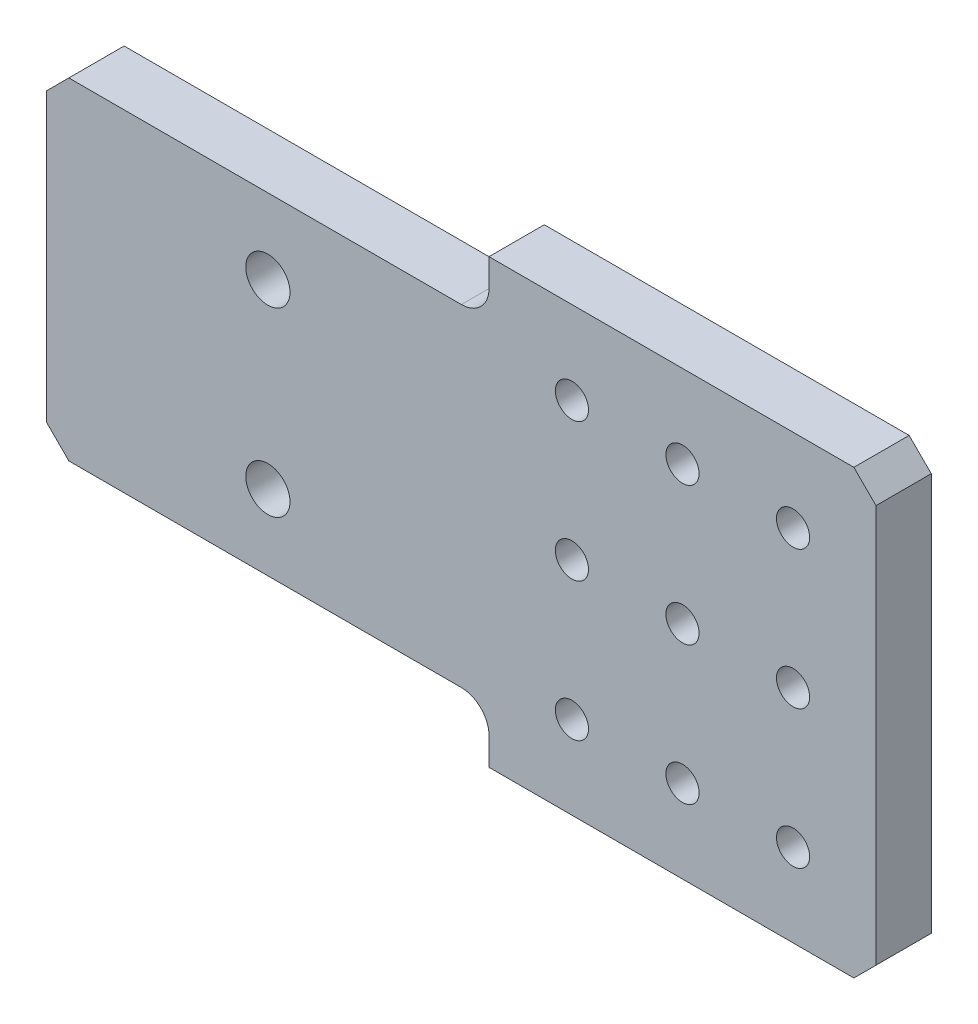
ISO-10303-21;
HEADER;
FILE_DESCRIPTION(('STEP AP214'),'2;1');
FILE_NAME('part.step','',(''),(''),'','','');
FILE_SCHEMA(('AUTOMOTIVE_DESIGN { 1 0 10303 214 1 1 1 1 }'));
ENDSEC;
DATA;
#1=APPLICATION_CONTEXT('core data for automotive mechanical design processes');
#2=APPLICATION_PROTOCOL_DEFINITION('international standard','automotive_design',2000,#1);
#3=PRODUCT_CONTEXT('',#1,'mechanical');
#4=PRODUCT('Part','Part','',(#3));
#5=PRODUCT_RELATED_PRODUCT_CATEGORY('part','',(#4));
#6=PRODUCT_DEFINITION_FORMATION('','',#4);
#7=PRODUCT_DEFINITION_CONTEXT('part definition',#1,'design');
#8=PRODUCT_DEFINITION('design','',#6,#7);
#9=PRODUCT_DEFINITION_SHAPE('','',#8);
#10=(LENGTH_UNIT() NAMED_UNIT(*) SI_UNIT(.MILLI.,.METRE.));
#11=(NAMED_UNIT(*) PLANE_ANGLE_UNIT() SI_UNIT($,.RADIAN.));
#12=(NAMED_UNIT(*) SI_UNIT($,.STERADIAN.) SOLID_ANGLE_UNIT());
#13=UNCERTAINTY_MEASURE_WITH_UNIT(LENGTH_MEASURE(1.E-05),#10,'distance_accuracy_value','');
#14=(GEOMETRIC_REPRESENTATION_CONTEXT(3) GLOBAL_UNCERTAINTY_ASSIGNED_CONTEXT((#13)) GLOBAL_UNIT_ASSIGNED_CONTEXT((#10,
#11,#12)) REPRESENTATION_CONTEXT('',''));
#15=CARTESIAN_POINT('',(0.,0.,0.));
#16=DIRECTION('',(0.,0.,1.));
#17=DIRECTION('',(1.,0.,0.));
#18=AXIS2_PLACEMENT_3D('',#15,#16,#17);
#19=CARTESIAN_POINT('',(3.75,1.75,0.5));
#20=DIRECTION('',(0.,0.,-1.));
#21=DIRECTION('',(-1.,0.,0.));
#22=AXIS2_PLACEMENT_3D('',#19,#20,#21);
#23=CYLINDRICAL_SURFACE('',#22,0.25);
#24=CARTESIAN_POINT('',(3.75,1.75,0.));
#25=DIRECTION('',(0.,0.,1.));
#26=DIRECTION('',(1.,0.,0.));
#27=AXIS2_PLACEMENT_3D('',#24,#25,#26);
#28=CIRCLE('',#27,0.25);
#29=CARTESIAN_POINT('',(3.75,1.5,0.));
#30=VERTEX_POINT('',#29);
#31=CARTESIAN_POINT('',(4.,1.75,0.));
#32=VERTEX_POINT('',#31);
#33=EDGE_CURVE('E168',#30,#32,#28,.T.);
#34=ORIENTED_EDGE('',*,*,#33,.F.);
#35=DIRECTION('',(0.,0.,-1.));
#36=VECTOR('',#35,1.);
#37=CARTESIAN_POINT('',(3.75,1.5,0.5));
#38=LINE('',#37,#36);
#39=CARTESIAN_POINT('',(3.75,1.5,0.5));
#40=VERTEX_POINT('',#39);
#41=EDGE_CURVE('E156',#40,#30,#38,.T.);
#42=ORIENTED_EDGE('',*,*,#41,.F.);
#43=CARTESIAN_POINT('',(3.75,1.75,0.5));
#44=DIRECTION('',(0.,0.,1.));
#45=DIRECTION('',(1.,0.,0.));
#46=AXIS2_PLACEMENT_3D('',#43,#44,#45);
#47=CIRCLE('',#46,0.25);
#48=CARTESIAN_POINT('',(4.,1.75,0.5));
#49=VERTEX_POINT('',#48);
#50=EDGE_CURVE('E163',#40,#49,#47,.T.);
#51=ORIENTED_EDGE('',*,*,#50,.T.);
#52=DIRECTION('',(0.,0.,-1.));
#53=VECTOR('',#52,1.);
#54=CARTESIAN_POINT('',(4.,1.75,0.5));
#55=LINE('',#54,#53);
#56=EDGE_CURVE('E201',#49,#32,#55,.T.);
#57=ORIENTED_EDGE('',*,*,#56,.T.);
#58=EDGE_LOOP('',(#34,#42,#51,#57));
#59=FACE_BOUND('',#58,.T.);
#60=ADVANCED_FACE('F47',(#59),#23,.F.);
#61=CARTESIAN_POINT('',(0.,1.5,0.5));
#62=DIRECTION('',(0.,1.,0.));
#63=DIRECTION('',(0.,0.,1.));
#64=AXIS2_PLACEMENT_3D('',#61,#62,#63);
#65=PLANE('',#64);
#66=DIRECTION('',(1.,0.,0.));
#67=VECTOR('',#66,1.);
#68=CARTESIAN_POINT('',(0.,1.5,0.));
#69=LINE('',#68,#67);
#70=CARTESIAN_POINT('',(0.199999999999999,1.5,0.));
#71=VERTEX_POINT('',#70);
#72=EDGE_CURVE('E202',#71,#30,#69,.T.);
#73=ORIENTED_EDGE('',*,*,#72,.F.);
#74=DIRECTION('',(0.,0.,1.));
#75=VECTOR('',#74,1.);
#76=CARTESIAN_POINT('',(0.199999999999999,1.5,0.5));
#77=LINE('',#76,#75);
#78=CARTESIAN_POINT('',(0.199999999999999,1.5,0.5));
#79=VERTEX_POINT('',#78);
#80=EDGE_CURVE('E157',#71,#79,#77,.T.);
#81=ORIENTED_EDGE('',*,*,#80,.T.);
#82=DIRECTION('',(1.,0.,0.));
#83=VECTOR('',#82,1.);
#84=CARTESIAN_POINT('',(0.,1.5,0.5));
#85=LINE('',#84,#83);
#86=EDGE_CURVE('E155',#79,#40,#85,.T.);
#87=ORIENTED_EDGE('',*,*,#86,.T.);
#88=ORIENTED_EDGE('',*,*,#41,.T.);
#89=EDGE_LOOP('',(#73,#81,#87,#88));
#90=FACE_BOUND('',#89,.T.);
#91=ADVANCED_FACE('F154',(#90),#65,.T.);
#92=CARTESIAN_POINT('',(0.,0.,0.5));
#93=DIRECTION('',(-1.,0.,0.));
#94=DIRECTION('',(0.,0.,1.));
#95=AXIS2_PLACEMENT_3D('',#92,#93,#94);
#96=PLANE('',#95);
#97=DIRECTION('',(0.,1.,0.));
#98=VECTOR('',#97,1.);
#99=CARTESIAN_POINT('',(0.,0.,0.));
#100=LINE('',#99,#98);
#101=CARTESIAN_POINT('',(0.,-1.3,0.));
#102=VERTEX_POINT('',#101);
#103=CARTESIAN_POINT('',(0.,1.3,0.));
#104=VERTEX_POINT('',#103);
#105=EDGE_CURVE('E208',#102,#104,#100,.T.);
#106=ORIENTED_EDGE('',*,*,#105,.F.);
#107=DIRECTION('',(0.,0.,1.));
#108=VECTOR('',#107,1.);
#109=CARTESIAN_POINT('',(0.,-1.3,0.5));
#110=LINE('',#109,#108);
#111=CARTESIAN_POINT('',(0.,-1.3,0.5));
#112=VERTEX_POINT('',#111);
#113=EDGE_CURVE('E11',#102,#112,#110,.T.);
#114=ORIENTED_EDGE('',*,*,#113,.T.);
#115=DIRECTION('',(0.,1.,0.));
#116=VECTOR('',#115,1.);
#117=CARTESIAN_POINT('',(0.,0.,0.5));
#118=LINE('',#117,#116);
#119=CARTESIAN_POINT('',(0.,1.3,0.5));
#120=VERTEX_POINT('',#119);
#121=EDGE_CURVE('E162',#112,#120,#118,.T.);
#122=ORIENTED_EDGE('',*,*,#121,.T.);
#123=DIRECTION('',(0.,0.,-1.));
#124=VECTOR('',#123,1.);
#125=CARTESIAN_POINT('',(0.,1.3,0.5));
#126=LINE('',#125,#124);
#127=EDGE_CURVE('E173',#120,#104,#126,.T.);
#128=ORIENTED_EDGE('',*,*,#127,.T.);
#129=EDGE_LOOP('',(#106,#114,#122,#128));
#130=FACE_BOUND('',#129,.T.);
#131=ADVANCED_FACE('F399',(#130),#96,.T.);
#132=CARTESIAN_POINT('',(0.,-1.5,0.5));
#133=DIRECTION('',(0.,1.,0.));
#134=DIRECTION('',(0.,0.,1.));
#135=AXIS2_PLACEMENT_3D('',#132,#133,#134);
#136=PLANE('',#135);
#137=DIRECTION('',(1.,0.,0.));
#138=VECTOR('',#137,1.);
#139=CARTESIAN_POINT('',(0.,-1.5,0.5));
#140=LINE('',#139,#138);
#141=CARTESIAN_POINT('',(0.200000000000001,-1.5,0.5));
#142=VERTEX_POINT('',#141);
#143=CARTESIAN_POINT('',(3.75,-1.5,0.5));
#144=VERTEX_POINT('',#143);
#145=EDGE_CURVE('E187',#142,#144,#140,.T.);
#146=ORIENTED_EDGE('',*,*,#145,.F.);
#147=DIRECTION('',(0.,0.,-1.));
#148=VECTOR('',#147,1.);
#149=CARTESIAN_POINT('',(0.200000000000001,-1.5,0.));
#150=LINE('',#149,#148);
#151=CARTESIAN_POINT('',(0.200000000000001,-1.5,0.));
#152=VERTEX_POINT('',#151);
#153=EDGE_CURVE('E56',#142,#152,#150,.T.);
#154=ORIENTED_EDGE('',*,*,#153,.T.);
#155=DIRECTION('',(1.,0.,0.));
#156=VECTOR('',#155,1.);
#157=CARTESIAN_POINT('',(0.,-1.5,0.));
#158=LINE('',#157,#156);
#159=CARTESIAN_POINT('',(3.75,-1.5,0.));
#160=VERTEX_POINT('',#159);
#161=EDGE_CURVE('E209',#152,#160,#158,.T.);
#162=ORIENTED_EDGE('',*,*,#161,.T.);
#163=DIRECTION('',(0.,0.,-1.));
#164=VECTOR('',#163,1.);
#165=CARTESIAN_POINT('',(3.75,-1.5,0.5));
#166=LINE('',#165,#164);
#167=EDGE_CURVE('E174',#144,#160,#166,.T.);
#168=ORIENTED_EDGE('',*,*,#167,.F.);
#169=EDGE_LOOP('',(#146,#154,#162,#168));
#170=FACE_BOUND('',#169,.T.);
#171=ADVANCED_FACE('F396',(#170),#136,.F.);
#172=CARTESIAN_POINT('',(3.75,-1.75,0.5));
#173=DIRECTION('',(0.,0.,-1.));
#174=DIRECTION('',(-1.,0.,0.));
#175=AXIS2_PLACEMENT_3D('',#172,#173,#174);
#176=CYLINDRICAL_SURFACE('',#175,0.25);
#177=CARTESIAN_POINT('',(3.75,-1.75,0.));
#178=DIRECTION('',(0.,0.,1.));
#179=DIRECTION('',(1.,0.,0.));
#180=AXIS2_PLACEMENT_3D('',#177,#178,#179);
#181=CIRCLE('',#180,0.25);
#182=CARTESIAN_POINT('',(4.,-1.75,0.));
#183=VERTEX_POINT('',#182);
#184=EDGE_CURVE('E215',#183,#160,#181,.T.);
#185=ORIENTED_EDGE('',*,*,#184,.F.);
#186=DIRECTION('',(0.,0.,-1.));
#187=VECTOR('',#186,1.);
#188=CARTESIAN_POINT('',(4.,-1.75,0.5));
#189=LINE('',#188,#187);
#190=CARTESIAN_POINT('',(4.,-1.75,0.5));
#191=VERTEX_POINT('',#190);
#192=EDGE_CURVE('E226',#191,#183,#189,.T.);
#193=ORIENTED_EDGE('',*,*,#192,.F.);
#194=CARTESIAN_POINT('',(3.75,-1.75,0.5));
#195=DIRECTION('',(0.,0.,1.));
#196=DIRECTION('',(1.,0.,0.));
#197=AXIS2_PLACEMENT_3D('',#194,#195,#196);
#198=CIRCLE('',#197,0.25);
#199=EDGE_CURVE('E186',#191,#144,#198,.T.);
#200=ORIENTED_EDGE('',*,*,#199,.T.);
#201=ORIENTED_EDGE('',*,*,#167,.T.);
#202=EDGE_LOOP('',(#185,#193,#200,#201));
#203=FACE_BOUND('',#202,.T.);
#204=ADVANCED_FACE('F392',(#203),#176,.F.);
#205=CARTESIAN_POINT('',(4.,0.,0.5));
#206=DIRECTION('',(1.,0.,0.));
#207=DIRECTION('',(0.,0.,-1.));
#208=AXIS2_PLACEMENT_3D('',#205,#206,#207);
#209=PLANE('',#208);
#210=DIRECTION('',(0.,-1.,0.));
#211=VECTOR('',#210,1.);
#212=CARTESIAN_POINT('',(4.,0.,0.));
#213=LINE('',#212,#211);
#214=CARTESIAN_POINT('',(4.,-2.,0.));
#215=VERTEX_POINT('',#214);
#216=EDGE_CURVE('E214',#183,#215,#213,.T.);
#217=ORIENTED_EDGE('',*,*,#216,.T.);
#218=DIRECTION('',(0.,0.,-1.));
#219=VECTOR('',#218,1.);
#220=CARTESIAN_POINT('',(4.,-2.,0.5));
#221=LINE('',#220,#219);
#222=CARTESIAN_POINT('',(4.,-2.,0.5));
#223=VERTEX_POINT('',#222);
#224=EDGE_CURVE('E229',#223,#215,#221,.T.);
#225=ORIENTED_EDGE('',*,*,#224,.F.);
#226=DIRECTION('',(0.,-1.,0.));
#227=VECTOR('',#226,1.);
#228=CARTESIAN_POINT('',(4.,0.,0.5));
#229=LINE('',#228,#227);
#230=EDGE_CURVE('E192',#191,#223,#229,.T.);
#231=ORIENTED_EDGE('',*,*,#230,.F.);
#232=ORIENTED_EDGE('',*,*,#192,.T.);
#233=EDGE_LOOP('',(#217,#225,#231,#232));
#234=FACE_BOUND('',#233,.T.);
#235=ADVANCED_FACE('F389',(#234),#209,.F.);
#236=CARTESIAN_POINT('',(0.,-2.,0.5));
#237=DIRECTION('',(0.,-1.,0.));
#238=DIRECTION('',(0.,0.,-1.));
#239=AXIS2_PLACEMENT_3D('',#236,#237,#238);
#240=PLANE('',#239);
#241=DIRECTION('',(-1.,0.,0.));
#242=VECTOR('',#241,1.);
#243=CARTESIAN_POINT('',(0.,-2.,0.));
#244=LINE('',#243,#242);
#245=CARTESIAN_POINT('',(7.3,-2.,0.));
#246=VERTEX_POINT('',#245);
#247=EDGE_CURVE('E217',#246,#215,#244,.T.);
#248=ORIENTED_EDGE('',*,*,#247,.F.);
#249=DIRECTION('',(0.,0.,1.));
#250=VECTOR('',#249,1.);
#251=CARTESIAN_POINT('',(7.3,-2.,0.5));
#252=LINE('',#251,#250);
#253=CARTESIAN_POINT('',(7.3,-2.,0.5));
#254=VERTEX_POINT('',#253);
#255=EDGE_CURVE('E259',#246,#254,#252,.T.);
#256=ORIENTED_EDGE('',*,*,#255,.T.);
#257=DIRECTION('',(-1.,0.,0.));
#258=VECTOR('',#257,1.);
#259=CARTESIAN_POINT('',(0.,-2.,0.5));
#260=LINE('',#259,#258);
#261=EDGE_CURVE('E198',#254,#223,#260,.T.);
#262=ORIENTED_EDGE('',*,*,#261,.T.);
#263=ORIENTED_EDGE('',*,*,#224,.T.);
#264=EDGE_LOOP('',(#248,#256,#262,#263));
#265=FACE_BOUND('',#264,.T.);
#266=ADVANCED_FACE('F382',(#265),#240,.T.);
#267=CARTESIAN_POINT('',(7.5,0.,0.5));
#268=DIRECTION('',(-1.,0.,0.));
#269=DIRECTION('',(0.,0.,1.));
#270=AXIS2_PLACEMENT_3D('',#267,#268,#269);
#271=PLANE('',#270);
#272=DIRECTION('',(0.,1.,0.));
#273=VECTOR('',#272,1.);
#274=CARTESIAN_POINT('',(7.5,0.,0.5));
#275=LINE('',#274,#273);
#276=CARTESIAN_POINT('',(7.5,-1.8,0.5));
#277=VERTEX_POINT('',#276);
#278=CARTESIAN_POINT('',(7.5,1.8,0.5));
#279=VERTEX_POINT('',#278);
#280=EDGE_CURVE('E196',#277,#279,#275,.T.);
#281=ORIENTED_EDGE('',*,*,#280,.F.);
#282=DIRECTION('',(0.,0.,-1.));
#283=VECTOR('',#282,1.);
#284=CARTESIAN_POINT('',(7.5,-1.8,0.));
#285=LINE('',#284,#283);
#286=CARTESIAN_POINT('',(7.5,-1.8,0.));
#287=VERTEX_POINT('',#286);
#288=EDGE_CURVE('E252',#277,#287,#285,.T.);
#289=ORIENTED_EDGE('',*,*,#288,.T.);
#290=DIRECTION('',(0.,1.,0.));
#291=VECTOR('',#290,1.);
#292=CARTESIAN_POINT('',(7.5,0.,0.));
#293=LINE('',#292,#291);
#294=CARTESIAN_POINT('',(7.5,1.8,0.));
#295=VERTEX_POINT('',#294);
#296=EDGE_CURVE('E219',#287,#295,#293,.T.);
#297=ORIENTED_EDGE('',*,*,#296,.T.);
#298=DIRECTION('',(0.,0.,1.));
#299=VECTOR('',#298,1.);
#300=CARTESIAN_POINT('',(7.5,1.8,0.5));
#301=LINE('',#300,#299);
#302=EDGE_CURVE('E248',#295,#279,#301,.T.);
#303=ORIENTED_EDGE('',*,*,#302,.T.);
#304=EDGE_LOOP('',(#281,#289,#297,#303));
#305=FACE_BOUND('',#304,.T.);
#306=ADVANCED_FACE('F374',(#305),#271,.F.);
#307=CARTESIAN_POINT('',(0.,2.,0.5));
#308=DIRECTION('',(0.,-1.,0.));
#309=DIRECTION('',(0.,0.,-1.));
#310=AXIS2_PLACEMENT_3D('',#307,#308,#309);
#311=PLANE('',#310);
#312=DIRECTION('',(-1.,0.,0.));
#313=VECTOR('',#312,1.);
#314=CARTESIAN_POINT('',(0.,2.,0.5));
#315=LINE('',#314,#313);
#316=CARTESIAN_POINT('',(7.3,2.,0.5));
#317=VERTEX_POINT('',#316);
#318=CARTESIAN_POINT('',(4.,2.,0.5));
#319=VERTEX_POINT('',#318);
#320=EDGE_CURVE('E199',#317,#319,#315,.T.);
#321=ORIENTED_EDGE('',*,*,#320,.F.);
#322=DIRECTION('',(0.,0.,-1.));
#323=VECTOR('',#322,1.);
#324=CARTESIAN_POINT('',(7.3,2.,0.5));
#325=LINE('',#324,#323);
#326=CARTESIAN_POINT('',(7.3,2.,0.));
#327=VERTEX_POINT('',#326);
#328=EDGE_CURVE('E246',#317,#327,#325,.T.);
#329=ORIENTED_EDGE('',*,*,#328,.T.);
#330=DIRECTION('',(-1.,0.,0.));
#331=VECTOR('',#330,1.);
#332=CARTESIAN_POINT('',(0.,2.,0.));
#333=LINE('',#332,#331);
#334=CARTESIAN_POINT('',(4.,2.,0.));
#335=VERTEX_POINT('',#334);
#336=EDGE_CURVE('E182',#327,#335,#333,.T.);
#337=ORIENTED_EDGE('',*,*,#336,.T.);
#338=DIRECTION('',(0.,0.,-1.));
#339=VECTOR('',#338,1.);
#340=CARTESIAN_POINT('',(4.,2.,0.5));
#341=LINE('',#340,#339);
#342=EDGE_CURVE('E221',#319,#335,#341,.T.);
#343=ORIENTED_EDGE('',*,*,#342,.F.);
#344=EDGE_LOOP('',(#321,#329,#337,#343));
#345=FACE_BOUND('',#344,.T.);
#346=ADVANCED_FACE('F439',(#345),#311,.F.);
#347=CARTESIAN_POINT('',(4.,0.,0.5));
#348=DIRECTION('',(-1.,0.,0.));
#349=DIRECTION('',(0.,0.,1.));
#350=AXIS2_PLACEMENT_3D('',#347,#348,#349);
#351=PLANE('',#350);
#352=DIRECTION('',(0.,1.,0.));
#353=VECTOR('',#352,1.);
#354=CARTESIAN_POINT('',(4.,0.,0.));
#355=LINE('',#354,#353);
#356=EDGE_CURVE('E177',#32,#335,#355,.T.);
#357=ORIENTED_EDGE('',*,*,#356,.F.);
#358=ORIENTED_EDGE('',*,*,#56,.F.);
#359=DIRECTION('',(0.,1.,0.));
#360=VECTOR('',#359,1.);
#361=CARTESIAN_POINT('',(4.,0.,0.5));
#362=LINE('',#361,#360);
#363=EDGE_CURVE('E180',#49,#319,#362,.T.);
#364=ORIENTED_EDGE('',*,*,#363,.T.);
#365=ORIENTED_EDGE('',*,*,#342,.T.);
#366=EDGE_LOOP('',(#357,#358,#364,#365));
#367=FACE_BOUND('',#366,.T.);
#368=ADVANCED_FACE('F336',(#367),#351,.T.);
#369=CARTESIAN_POINT('',(0.,0.,0.5));
#370=DIRECTION('',(0.,0.,1.));
#371=DIRECTION('',(1.,0.,0.));
#372=AXIS2_PLACEMENT_3D('',#369,#370,#371);
#373=PLANE('',#372);
#374=CARTESIAN_POINT('',(5.75,1.25,0.5));
#375=DIRECTION('',(0.,0.,1.));
#376=DIRECTION('',(1.,0.,0.));
#377=AXIS2_PLACEMENT_3D('',#374,#375,#376);
#378=CIRCLE('',#377,0.15);
#379=CARTESIAN_POINT('',(5.9,1.25,0.5));
#380=VERTEX_POINT('',#379);
#381=EDGE_CURVE('E310',#380,#380,#378,.T.);
#382=ORIENTED_EDGE('',*,*,#381,.F.);
#383=EDGE_LOOP('',(#382));
#384=FACE_BOUND('',#383,.T.);
#385=CARTESIAN_POINT('',(6.75,1.25,0.5));
#386=DIRECTION('',(0.,0.,1.));
#387=DIRECTION('',(1.,0.,0.));
#388=AXIS2_PLACEMENT_3D('',#385,#386,#387);
#389=CIRCLE('',#388,0.15);
#390=CARTESIAN_POINT('',(6.9,1.25,0.5));
#391=VERTEX_POINT('',#390);
#392=EDGE_CURVE('E320',#391,#391,#389,.T.);
#393=ORIENTED_EDGE('',*,*,#392,.F.);
#394=EDGE_LOOP('',(#393));
#395=FACE_BOUND('',#394,.T.);
#396=CARTESIAN_POINT('',(6.75,0.,0.5));
#397=DIRECTION('',(0.,0.,1.));
#398=DIRECTION('',(1.,0.,0.));
#399=AXIS2_PLACEMENT_3D('',#396,#397,#398);
#400=CIRCLE('',#399,0.15);
#401=CARTESIAN_POINT('',(6.9,0.,0.5));
#402=VERTEX_POINT('',#401);
#403=EDGE_CURVE('E311',#402,#402,#400,.T.);
#404=ORIENTED_EDGE('',*,*,#403,.F.);
#405=EDGE_LOOP('',(#404));
#406=FACE_BOUND('',#405,.T.);
#407=CARTESIAN_POINT('',(6.75,-1.25,0.5));
#408=DIRECTION('',(0.,0.,1.));
#409=DIRECTION('',(1.,0.,0.));
#410=AXIS2_PLACEMENT_3D('',#407,#408,#409);
#411=CIRCLE('',#410,0.15);
#412=CARTESIAN_POINT('',(6.9,-1.25,0.5));
#413=VERTEX_POINT('',#412);
#414=EDGE_CURVE('E309',#413,#413,#411,.T.);
#415=ORIENTED_EDGE('',*,*,#414,.F.);
#416=EDGE_LOOP('',(#415));
#417=FACE_BOUND('',#416,.T.);
#418=CARTESIAN_POINT('',(5.75,-1.25,0.5));
#419=DIRECTION('',(0.,0.,1.));
#420=DIRECTION('',(1.,0.,0.));
#421=AXIS2_PLACEMENT_3D('',#418,#419,#420);
#422=CIRCLE('',#421,0.15);
#423=CARTESIAN_POINT('',(5.9,-1.25,0.5));
#424=VERTEX_POINT('',#423);
#425=EDGE_CURVE('E314',#424,#424,#422,.T.);
#426=ORIENTED_EDGE('',*,*,#425,.F.);
#427=EDGE_LOOP('',(#426));
#428=FACE_BOUND('',#427,.T.);
#429=CARTESIAN_POINT('',(4.75,-1.25,0.5));
#430=DIRECTION('',(0.,0.,1.));
#431=DIRECTION('',(1.,0.,0.));
#432=AXIS2_PLACEMENT_3D('',#429,#430,#431);
#433=CIRCLE('',#432,0.15);
#434=CARTESIAN_POINT('',(4.9,-1.25,0.5));
#435=VERTEX_POINT('',#434);
#436=EDGE_CURVE('E327',#435,#435,#433,.T.);
#437=ORIENTED_EDGE('',*,*,#436,.F.);
#438=EDGE_LOOP('',(#437));
#439=FACE_BOUND('',#438,.T.);
#440=CARTESIAN_POINT('',(4.75,0.,0.5));
#441=DIRECTION('',(0.,0.,1.));
#442=DIRECTION('',(1.,0.,0.));
#443=AXIS2_PLACEMENT_3D('',#440,#441,#442);
#444=CIRCLE('',#443,0.15);
#445=CARTESIAN_POINT('',(4.9,0.,0.5));
#446=VERTEX_POINT('',#445);
#447=EDGE_CURVE('E324',#446,#446,#444,.T.);
#448=ORIENTED_EDGE('',*,*,#447,.F.);
#449=EDGE_LOOP('',(#448));
#450=FACE_BOUND('',#449,.T.);
#451=CARTESIAN_POINT('',(5.75,0.,0.5));
#452=DIRECTION('',(0.,0.,1.));
#453=DIRECTION('',(1.,0.,0.));
#454=AXIS2_PLACEMENT_3D('',#451,#452,#453);
#455=CIRCLE('',#454,0.15);
#456=CARTESIAN_POINT('',(5.9,0.,0.5));
#457=VERTEX_POINT('',#456);
#458=EDGE_CURVE('E325',#457,#457,#455,.T.);
#459=ORIENTED_EDGE('',*,*,#458,.F.);
#460=EDGE_LOOP('',(#459));
#461=FACE_BOUND('',#460,.T.);
#462=CARTESIAN_POINT('',(4.75,1.25,0.5));
#463=DIRECTION('',(0.,0.,1.));
#464=DIRECTION('',(1.,0.,0.));
#465=AXIS2_PLACEMENT_3D('',#462,#463,#464);
#466=CIRCLE('',#465,0.15);
#467=CARTESIAN_POINT('',(4.9,1.25,0.5));
#468=VERTEX_POINT('',#467);
#469=EDGE_CURVE('E277',#468,#468,#466,.T.);
#470=ORIENTED_EDGE('',*,*,#469,.F.);
#471=EDGE_LOOP('',(#470));
#472=FACE_BOUND('',#471,.T.);
#473=CARTESIAN_POINT('',(2.,0.82,0.5));
#474=DIRECTION('',(0.,0.,1.));
#475=DIRECTION('',(1.,0.,0.));
#476=AXIS2_PLACEMENT_3D('',#473,#474,#475);
#477=CIRCLE('',#476,0.2);
#478=CARTESIAN_POINT('',(2.2,0.82,0.5));
#479=VERTEX_POINT('',#478);
#480=EDGE_CURVE('E267',#479,#479,#477,.T.);
#481=ORIENTED_EDGE('',*,*,#480,.F.);
#482=EDGE_LOOP('',(#481));
#483=FACE_BOUND('',#482,.T.);
#484=CARTESIAN_POINT('',(2.,-0.82,0.5));
#485=DIRECTION('',(0.,0.,1.));
#486=DIRECTION('',(1.,0.,0.));
#487=AXIS2_PLACEMENT_3D('',#484,#485,#486);
#488=CIRCLE('',#487,0.2);
#489=CARTESIAN_POINT('',(2.2,-0.82,0.5));
#490=VERTEX_POINT('',#489);
#491=EDGE_CURVE('E184',#490,#490,#488,.T.);
#492=ORIENTED_EDGE('',*,*,#491,.F.);
#493=EDGE_LOOP('',(#492));
#494=FACE_BOUND('',#493,.T.);
#495=ORIENTED_EDGE('',*,*,#261,.F.);
#496=DIRECTION('',(0.707106781186549,0.707106781186546,0.));
#497=VECTOR('',#496,1.);
#498=CARTESIAN_POINT('',(4.64999999999998,-4.65,0.5));
#499=LINE('',#498,#497);
#500=EDGE_CURVE('E265',#254,#277,#499,.T.);
#501=ORIENTED_EDGE('',*,*,#500,.T.);
#502=ORIENTED_EDGE('',*,*,#280,.T.);
#503=DIRECTION('',(0.707106781186546,-0.707106781186549,0.));
#504=VECTOR('',#503,1.);
#505=CARTESIAN_POINT('',(4.65000000000002,4.65,0.5));
#506=LINE('',#505,#504);
#507=EDGE_CURVE('E244',#279,#317,#506,.F.);
#508=ORIENTED_EDGE('',*,*,#507,.T.);
#509=ORIENTED_EDGE('',*,*,#320,.T.);
#510=ORIENTED_EDGE('',*,*,#363,.F.);
#511=ORIENTED_EDGE('',*,*,#50,.F.);
#512=ORIENTED_EDGE('',*,*,#86,.F.);
#513=DIRECTION('',(0.707106781186548,0.707106781186548,0.));
#514=VECTOR('',#513,1.);
#515=CARTESIAN_POINT('',(-0.65,0.65,0.5));
#516=LINE('',#515,#514);
#517=EDGE_CURVE('E245',#79,#120,#516,.F.);
#518=ORIENTED_EDGE('',*,*,#517,.T.);
#519=ORIENTED_EDGE('',*,*,#121,.F.);
#520=DIRECTION('',(0.707106781186546,-0.707106781186549,0.));
#521=VECTOR('',#520,1.);
#522=CARTESIAN_POINT('',(-0.649999999999999,-0.649999999999997,0.5));
#523=LINE('',#522,#521);
#524=EDGE_CURVE('E70',#112,#142,#523,.T.);
#525=ORIENTED_EDGE('',*,*,#524,.T.);
#526=ORIENTED_EDGE('',*,*,#145,.T.);
#527=ORIENTED_EDGE('',*,*,#199,.F.);
#528=ORIENTED_EDGE('',*,*,#230,.T.);
#529=EDGE_LOOP('',(#495,#501,#502,#508,#509,#510,#511,#512,#518,#519,#525,#526,#527,#528));
#530=FACE_BOUND('',#529,.T.);
#531=ADVANCED_FACE('F171',(#384,#395,#406,#417,#428,#439,#450,#461,#472,#483,#494,#530),#373,.T.);
#532=CARTESIAN_POINT('',(0.,0.,0.));
#533=DIRECTION('',(0.,0.,1.));
#534=DIRECTION('',(1.,0.,0.));
#535=AXIS2_PLACEMENT_3D('',#532,#533,#534);
#536=PLANE('',#535);
#537=CARTESIAN_POINT('',(5.75,1.25,0.));
#538=DIRECTION('',(0.,0.,1.));
#539=DIRECTION('',(1.,0.,0.));
#540=AXIS2_PLACEMENT_3D('',#537,#538,#539);
#541=CIRCLE('',#540,0.15);
#542=CARTESIAN_POINT('',(5.9,1.25,0.));
#543=VERTEX_POINT('',#542);
#544=EDGE_CURVE('E53',#543,#543,#541,.T.);
#545=ORIENTED_EDGE('',*,*,#544,.T.);
#546=EDGE_LOOP('',(#545));
#547=FACE_BOUND('',#546,.T.);
#548=CARTESIAN_POINT('',(6.75,1.25,0.));
#549=DIRECTION('',(0.,0.,1.));
#550=DIRECTION('',(1.,0.,0.));
#551=AXIS2_PLACEMENT_3D('',#548,#549,#550);
#552=CIRCLE('',#551,0.15);
#553=CARTESIAN_POINT('',(6.9,1.25,0.));
#554=VERTEX_POINT('',#553);
#555=EDGE_CURVE('E291',#554,#554,#552,.T.);
#556=ORIENTED_EDGE('',*,*,#555,.T.);
#557=EDGE_LOOP('',(#556));
#558=FACE_BOUND('',#557,.T.);
#559=CARTESIAN_POINT('',(6.75,0.,0.));
#560=DIRECTION('',(0.,0.,1.));
#561=DIRECTION('',(1.,0.,0.));
#562=AXIS2_PLACEMENT_3D('',#559,#560,#561);
#563=CIRCLE('',#562,0.15);
#564=CARTESIAN_POINT('',(6.9,0.,0.));
#565=VERTEX_POINT('',#564);
#566=EDGE_CURVE('E292',#565,#565,#563,.T.);
#567=ORIENTED_EDGE('',*,*,#566,.T.);
#568=EDGE_LOOP('',(#567));
#569=FACE_BOUND('',#568,.T.);
#570=CARTESIAN_POINT('',(6.75,-1.25,0.));
#571=DIRECTION('',(0.,0.,1.));
#572=DIRECTION('',(1.,0.,0.));
#573=AXIS2_PLACEMENT_3D('',#570,#571,#572);
#574=CIRCLE('',#573,0.15);
#575=CARTESIAN_POINT('',(6.9,-1.25,0.));
#576=VERTEX_POINT('',#575);
#577=EDGE_CURVE('E287',#576,#576,#574,.T.);
#578=ORIENTED_EDGE('',*,*,#577,.T.);
#579=EDGE_LOOP('',(#578));
#580=FACE_BOUND('',#579,.T.);
#581=CARTESIAN_POINT('',(5.75,-1.25,0.));
#582=DIRECTION('',(0.,0.,1.));
#583=DIRECTION('',(1.,0.,0.));
#584=AXIS2_PLACEMENT_3D('',#581,#582,#583);
#585=CIRCLE('',#584,0.15);
#586=CARTESIAN_POINT('',(5.9,-1.25,0.));
#587=VERTEX_POINT('',#586);
#588=EDGE_CURVE('E281',#587,#587,#585,.T.);
#589=ORIENTED_EDGE('',*,*,#588,.T.);
#590=EDGE_LOOP('',(#589));
#591=FACE_BOUND('',#590,.T.);
#592=CARTESIAN_POINT('',(4.75,-1.25,0.));
#593=DIRECTION('',(0.,0.,1.));
#594=DIRECTION('',(1.,0.,0.));
#595=AXIS2_PLACEMENT_3D('',#592,#593,#594);
#596=CIRCLE('',#595,0.15);
#597=CARTESIAN_POINT('',(4.9,-1.25,0.));
#598=VERTEX_POINT('',#597);
#599=EDGE_CURVE('E284',#598,#598,#596,.T.);
#600=ORIENTED_EDGE('',*,*,#599,.T.);
#601=EDGE_LOOP('',(#600));
#602=FACE_BOUND('',#601,.T.);
#603=CARTESIAN_POINT('',(4.75,0.,0.));
#604=DIRECTION('',(0.,0.,1.));
#605=DIRECTION('',(1.,0.,0.));
#606=AXIS2_PLACEMENT_3D('',#603,#604,#605);
#607=CIRCLE('',#606,0.15);
#608=CARTESIAN_POINT('',(4.9,0.,0.));
#609=VERTEX_POINT('',#608);
#610=EDGE_CURVE('E276',#609,#609,#607,.T.);
#611=ORIENTED_EDGE('',*,*,#610,.T.);
#612=EDGE_LOOP('',(#611));
#613=FACE_BOUND('',#612,.T.);
#614=CARTESIAN_POINT('',(5.75,0.,0.));
#615=DIRECTION('',(0.,0.,1.));
#616=DIRECTION('',(1.,0.,0.));
#617=AXIS2_PLACEMENT_3D('',#614,#615,#616);
#618=CIRCLE('',#617,0.15);
#619=CARTESIAN_POINT('',(5.9,0.,0.));
#620=VERTEX_POINT('',#619);
#621=EDGE_CURVE('E274',#620,#620,#618,.T.);
#622=ORIENTED_EDGE('',*,*,#621,.T.);
#623=EDGE_LOOP('',(#622));
#624=FACE_BOUND('',#623,.T.);
#625=CARTESIAN_POINT('',(4.75,1.25,0.));
#626=DIRECTION('',(0.,0.,1.));
#627=DIRECTION('',(1.,0.,0.));
#628=AXIS2_PLACEMENT_3D('',#625,#626,#627);
#629=CIRCLE('',#628,0.15);
#630=CARTESIAN_POINT('',(4.9,1.25,0.));
#631=VERTEX_POINT('',#630);
#632=EDGE_CURVE('E275',#631,#631,#629,.T.);
#633=ORIENTED_EDGE('',*,*,#632,.T.);
#634=EDGE_LOOP('',(#633));
#635=FACE_BOUND('',#634,.T.);
#636=CARTESIAN_POINT('',(2.,0.82,0.));
#637=DIRECTION('',(0.,0.,1.));
#638=DIRECTION('',(1.,0.,0.));
#639=AXIS2_PLACEMENT_3D('',#636,#637,#638);
#640=CIRCLE('',#639,0.2);
#641=CARTESIAN_POINT('',(2.2,0.82,0.));
#642=VERTEX_POINT('',#641);
#643=EDGE_CURVE('E206',#642,#642,#640,.T.);
#644=ORIENTED_EDGE('',*,*,#643,.T.);
#645=EDGE_LOOP('',(#644));
#646=FACE_BOUND('',#645,.T.);
#647=CARTESIAN_POINT('',(2.,-0.82,0.));
#648=DIRECTION('',(0.,0.,1.));
#649=DIRECTION('',(1.,0.,0.));
#650=AXIS2_PLACEMENT_3D('',#647,#648,#649);
#651=CIRCLE('',#650,0.2);
#652=CARTESIAN_POINT('',(2.2,-0.82,0.));
#653=VERTEX_POINT('',#652);
#654=EDGE_CURVE('E266',#653,#653,#651,.T.);
#655=ORIENTED_EDGE('',*,*,#654,.T.);
#656=EDGE_LOOP('',(#655));
#657=FACE_BOUND('',#656,.T.);
#658=ORIENTED_EDGE('',*,*,#296,.F.);
#659=DIRECTION('',(-0.707106781186549,-0.707106781186546,0.));
#660=VECTOR('',#659,1.);
#661=CARTESIAN_POINT('',(7.5,-1.8,0.));
#662=LINE('',#661,#660);
#663=EDGE_CURVE('E260',#287,#246,#662,.T.);
#664=ORIENTED_EDGE('',*,*,#663,.T.);
#665=ORIENTED_EDGE('',*,*,#247,.T.);
#666=ORIENTED_EDGE('',*,*,#216,.F.);
#667=ORIENTED_EDGE('',*,*,#184,.T.);
#668=ORIENTED_EDGE('',*,*,#161,.F.);
#669=DIRECTION('',(-0.707106781186546,0.707106781186549,0.));
#670=VECTOR('',#669,1.);
#671=CARTESIAN_POINT('',(0.200000000000001,-1.5,0.));
#672=LINE('',#671,#670);
#673=EDGE_CURVE('E254',#152,#102,#672,.T.);
#674=ORIENTED_EDGE('',*,*,#673,.T.);
#675=ORIENTED_EDGE('',*,*,#105,.T.);
#676=DIRECTION('',(-0.707106781186548,-0.707106781186548,0.));
#677=VECTOR('',#676,1.);
#678=CARTESIAN_POINT('',(0.,1.3,0.));
#679=LINE('',#678,#677);
#680=EDGE_CURVE('E239',#104,#71,#679,.F.);
#681=ORIENTED_EDGE('',*,*,#680,.T.);
#682=ORIENTED_EDGE('',*,*,#72,.T.);
#683=ORIENTED_EDGE('',*,*,#33,.T.);
#684=ORIENTED_EDGE('',*,*,#356,.T.);
#685=ORIENTED_EDGE('',*,*,#336,.F.);
#686=DIRECTION('',(-0.707106781186546,0.707106781186549,0.));
#687=VECTOR('',#686,1.);
#688=CARTESIAN_POINT('',(7.3,2.,0.));
#689=LINE('',#688,#687);
#690=EDGE_CURVE('E237',#327,#295,#689,.F.);
#691=ORIENTED_EDGE('',*,*,#690,.T.);
#692=EDGE_LOOP('',(#658,#664,#665,#666,#667,#668,#674,#675,#681,#682,#683,#684,#685,#691));
#693=FACE_BOUND('',#692,.T.);
#694=ADVANCED_FACE('F340',(#547,#558,#569,#580,#591,#602,#613,#624,#635,#646,#657,#693),#536,.F.);
#695=CARTESIAN_POINT('',(0.,1.3,0.5));
#696=DIRECTION('',(0.707106781186548,-0.707106781186548,0.));
#697=DIRECTION('',(0.,0.,-1.));
#698=AXIS2_PLACEMENT_3D('',#695,#696,#697);
#699=PLANE('',#698);
#700=ORIENTED_EDGE('',*,*,#517,.F.);
#701=ORIENTED_EDGE('',*,*,#80,.F.);
#702=ORIENTED_EDGE('',*,*,#680,.F.);
#703=ORIENTED_EDGE('',*,*,#127,.F.);
#704=EDGE_LOOP('',(#700,#701,#702,#703));
#705=FACE_BOUND('',#704,.T.);
#706=ADVANCED_FACE('F361',(#705),#699,.F.);
#707=CARTESIAN_POINT('',(7.3,2.,0.5));
#708=DIRECTION('',(-0.707106781186549,-0.707106781186546,0.));
#709=DIRECTION('',(0.,0.,-1.));
#710=AXIS2_PLACEMENT_3D('',#707,#708,#709);
#711=PLANE('',#710);
#712=ORIENTED_EDGE('',*,*,#507,.F.);
#713=ORIENTED_EDGE('',*,*,#302,.F.);
#714=ORIENTED_EDGE('',*,*,#690,.F.);
#715=ORIENTED_EDGE('',*,*,#328,.F.);
#716=EDGE_LOOP('',(#712,#713,#714,#715));
#717=FACE_BOUND('',#716,.T.);
#718=ADVANCED_FACE('F410',(#717),#711,.F.);
#719=CARTESIAN_POINT('',(7.5,-1.8,0.5));
#720=DIRECTION('',(0.707106781186546,-0.707106781186549,0.));
#721=DIRECTION('',(0.,0.,1.));
#722=AXIS2_PLACEMENT_3D('',#719,#720,#721);
#723=PLANE('',#722);
#724=ORIENTED_EDGE('',*,*,#500,.F.);
#725=ORIENTED_EDGE('',*,*,#255,.F.);
#726=ORIENTED_EDGE('',*,*,#663,.F.);
#727=ORIENTED_EDGE('',*,*,#288,.F.);
#728=EDGE_LOOP('',(#724,#725,#726,#727));
#729=FACE_BOUND('',#728,.T.);
#730=ADVANCED_FACE('F379',(#729),#723,.T.);
#731=CARTESIAN_POINT('',(0.200000000000001,-1.5,0.5));
#732=DIRECTION('',(-0.707106781186549,-0.707106781186546,0.));
#733=DIRECTION('',(0.,0.,1.));
#734=AXIS2_PLACEMENT_3D('',#731,#732,#733);
#735=PLANE('',#734);
#736=ORIENTED_EDGE('',*,*,#524,.F.);
#737=ORIENTED_EDGE('',*,*,#113,.F.);
#738=ORIENTED_EDGE('',*,*,#673,.F.);
#739=ORIENTED_EDGE('',*,*,#153,.F.);
#740=EDGE_LOOP('',(#736,#737,#738,#739));
#741=FACE_BOUND('',#740,.T.);
#742=ADVANCED_FACE('F55',(#741),#735,.T.);
#743=CARTESIAN_POINT('',(2.,-0.82,-0.5));
#744=DIRECTION('',(0.,0.,1.));
#745=DIRECTION('',(1.,0.,0.));
#746=AXIS2_PLACEMENT_3D('',#743,#744,#745);
#747=CYLINDRICAL_SURFACE('',#746,0.2);
#748=ORIENTED_EDGE('',*,*,#491,.T.);
#749=EDGE_LOOP('',(#748));
#750=FACE_BOUND('',#749,.T.);
#751=ORIENTED_EDGE('',*,*,#654,.F.);
#752=EDGE_LOOP('',(#751));
#753=FACE_BOUND('',#752,.T.);
#754=ADVANCED_FACE('F401',(#750,#753),#747,.F.);
#755=CARTESIAN_POINT('',(2.,0.82,-0.5));
#756=DIRECTION('',(0.,0.,1.));
#757=DIRECTION('',(1.,0.,0.));
#758=AXIS2_PLACEMENT_3D('',#755,#756,#757);
#759=CYLINDRICAL_SURFACE('',#758,0.2);
#760=ORIENTED_EDGE('',*,*,#480,.T.);
#761=EDGE_LOOP('',(#760));
#762=FACE_BOUND('',#761,.T.);
#763=ORIENTED_EDGE('',*,*,#643,.F.);
#764=EDGE_LOOP('',(#763));
#765=FACE_BOUND('',#764,.T.);
#766=ADVANCED_FACE('F360',(#762,#765),#759,.F.);
#767=CARTESIAN_POINT('',(4.75,1.25,-0.5));
#768=DIRECTION('',(0.,0.,1.));
#769=DIRECTION('',(1.,0.,0.));
#770=AXIS2_PLACEMENT_3D('',#767,#768,#769);
#771=CYLINDRICAL_SURFACE('',#770,0.15);
#772=ORIENTED_EDGE('',*,*,#469,.T.);
#773=EDGE_LOOP('',(#772));
#774=FACE_BOUND('',#773,.T.);
#775=ORIENTED_EDGE('',*,*,#632,.F.);
#776=EDGE_LOOP('',(#775));
#777=FACE_BOUND('',#776,.T.);
#778=ADVANCED_FACE('F352',(#774,#777),#771,.F.);
#779=CARTESIAN_POINT('',(5.75,0.,-0.5));
#780=DIRECTION('',(0.,0.,1.));
#781=DIRECTION('',(1.,0.,0.));
#782=AXIS2_PLACEMENT_3D('',#779,#780,#781);
#783=CYLINDRICAL_SURFACE('',#782,0.15);
#784=ORIENTED_EDGE('',*,*,#458,.T.);
#785=EDGE_LOOP('',(#784));
#786=FACE_BOUND('',#785,.T.);
#787=ORIENTED_EDGE('',*,*,#621,.F.);
#788=EDGE_LOOP('',(#787));
#789=FACE_BOUND('',#788,.T.);
#790=ADVANCED_FACE('F356',(#786,#789),#783,.F.);
#791=CARTESIAN_POINT('',(4.75,0.,-0.5));
#792=DIRECTION('',(0.,0.,1.));
#793=DIRECTION('',(1.,0.,0.));
#794=AXIS2_PLACEMENT_3D('',#791,#792,#793);
#795=CYLINDRICAL_SURFACE('',#794,0.15);
#796=ORIENTED_EDGE('',*,*,#447,.T.);
#797=EDGE_LOOP('',(#796));
#798=FACE_BOUND('',#797,.T.);
#799=ORIENTED_EDGE('',*,*,#610,.F.);
#800=EDGE_LOOP('',(#799));
#801=FACE_BOUND('',#800,.T.);
#802=ADVANCED_FACE('F551',(#798,#801),#795,.F.);
#803=CARTESIAN_POINT('',(4.75,-1.25,-0.5));
#804=DIRECTION('',(0.,0.,1.));
#805=DIRECTION('',(1.,0.,0.));
#806=AXIS2_PLACEMENT_3D('',#803,#804,#805);
#807=CYLINDRICAL_SURFACE('',#806,0.15);
#808=ORIENTED_EDGE('',*,*,#436,.T.);
#809=EDGE_LOOP('',(#808));
#810=FACE_BOUND('',#809,.T.);
#811=ORIENTED_EDGE('',*,*,#599,.F.);
#812=EDGE_LOOP('',(#811));
#813=FACE_BOUND('',#812,.T.);
#814=ADVANCED_FACE('F563',(#810,#813),#807,.F.);
#815=CARTESIAN_POINT('',(5.75,-1.25,-0.5));
#816=DIRECTION('',(0.,0.,1.));
#817=DIRECTION('',(1.,0.,0.));
#818=AXIS2_PLACEMENT_3D('',#815,#816,#817);
#819=CYLINDRICAL_SURFACE('',#818,0.15);
#820=ORIENTED_EDGE('',*,*,#425,.T.);
#821=EDGE_LOOP('',(#820));
#822=FACE_BOUND('',#821,.T.);
#823=ORIENTED_EDGE('',*,*,#588,.F.);
#824=EDGE_LOOP('',(#823));
#825=FACE_BOUND('',#824,.T.);
#826=ADVANCED_FACE('F331',(#822,#825),#819,.F.);
#827=CARTESIAN_POINT('',(6.75,-1.25,-0.5));
#828=DIRECTION('',(0.,0.,1.));
#829=DIRECTION('',(1.,0.,0.));
#830=AXIS2_PLACEMENT_3D('',#827,#828,#829);
#831=CYLINDRICAL_SURFACE('',#830,0.15);
#832=ORIENTED_EDGE('',*,*,#414,.T.);
#833=EDGE_LOOP('',(#832));
#834=FACE_BOUND('',#833,.T.);
#835=ORIENTED_EDGE('',*,*,#577,.F.);
#836=EDGE_LOOP('',(#835));
#837=FACE_BOUND('',#836,.T.);
#838=ADVANCED_FACE('F581',(#834,#837),#831,.F.);
#839=CARTESIAN_POINT('',(6.75,0.,-0.5));
#840=DIRECTION('',(0.,0.,1.));
#841=DIRECTION('',(1.,0.,0.));
#842=AXIS2_PLACEMENT_3D('',#839,#840,#841);
#843=CYLINDRICAL_SURFACE('',#842,0.15);
#844=ORIENTED_EDGE('',*,*,#403,.T.);
#845=EDGE_LOOP('',(#844));
#846=FACE_BOUND('',#845,.T.);
#847=ORIENTED_EDGE('',*,*,#566,.F.);
#848=EDGE_LOOP('',(#847));
#849=FACE_BOUND('',#848,.T.);
#850=ADVANCED_FACE('F595',(#846,#849),#843,.F.);
#851=CARTESIAN_POINT('',(6.75,1.25,-0.5));
#852=DIRECTION('',(0.,0.,1.));
#853=DIRECTION('',(1.,0.,0.));
#854=AXIS2_PLACEMENT_3D('',#851,#852,#853);
#855=CYLINDRICAL_SURFACE('',#854,0.15);
#856=ORIENTED_EDGE('',*,*,#392,.T.);
#857=EDGE_LOOP('',(#856));
#858=FACE_BOUND('',#857,.T.);
#859=ORIENTED_EDGE('',*,*,#555,.F.);
#860=EDGE_LOOP('',(#859));
#861=FACE_BOUND('',#860,.T.);
#862=ADVANCED_FACE('F605',(#858,#861),#855,.F.);
#863=CARTESIAN_POINT('',(5.75,1.25,-0.5));
#864=DIRECTION('',(0.,0.,1.));
#865=DIRECTION('',(1.,0.,0.));
#866=AXIS2_PLACEMENT_3D('',#863,#864,#865);
#867=CYLINDRICAL_SURFACE('',#866,0.15);
#868=ORIENTED_EDGE('',*,*,#381,.T.);
#869=EDGE_LOOP('',(#868));
#870=FACE_BOUND('',#869,.T.);
#871=ORIENTED_EDGE('',*,*,#544,.F.);
#872=EDGE_LOOP('',(#871));
#873=FACE_BOUND('',#872,.T.);
#874=ADVANCED_FACE('F614',(#870,#873),#867,.F.);
#875=CLOSED_SHELL('',(#60,#91,#131,#171,#204,#235,#266,#306,#346,#368,#531,#694,#706,#718,#730,
#742,#754,#766,#778,#790,#802,#814,#826,#838,#850,#862,#874));
#876=MANIFOLD_SOLID_BREP('B2',#875);
#877=ADVANCED_BREP_SHAPE_REPRESENTATION('',(#18,#876),#14);
#878=SHAPE_DEFINITION_REPRESENTATION(#9,#877);
ENDSEC;
END-ISO-10303-21;
